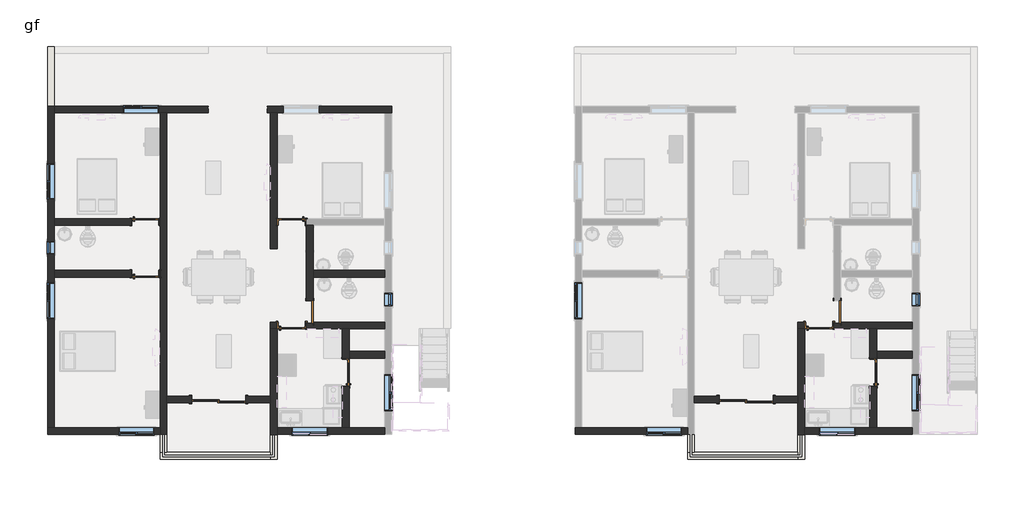
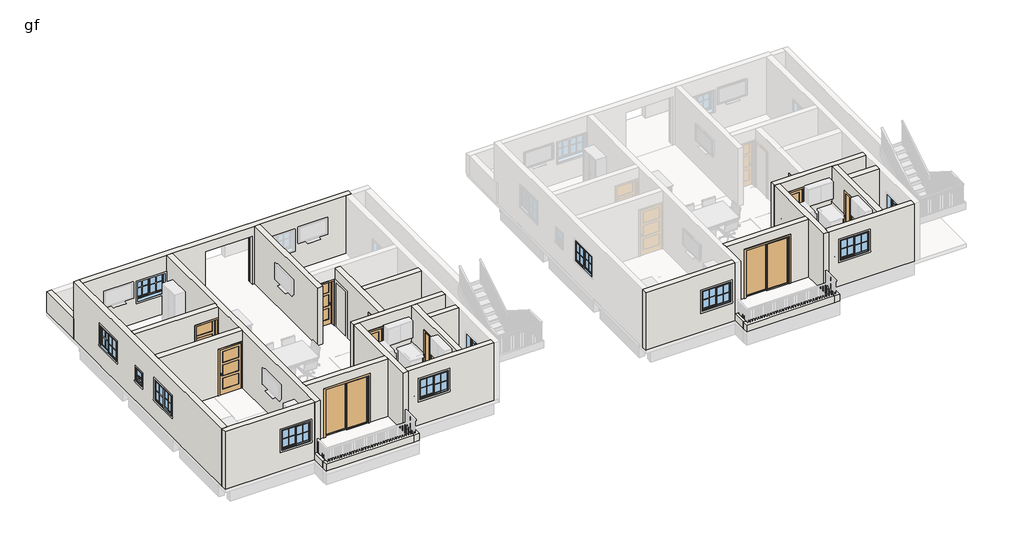
# One storey, part 1 of 8: 30 walls, 13 windows, 11 doors.
"""IFC4 building model written with IfcOpenShell, lengths in millimetres."""

from ifc_helpers import new_model, si_unit, frame, origin, place, context, project, spatial, polyline, outline, extrude, faceted_brep, transform, mapped, element, save
from components import door_d4d75d1e, door_2334f446, door_80766924, door_a1484949, window_608ea798, window_2eef0573, window_a5b1ea32

model = new_model("IFC4")

# Units and contexts
model_context = context("Model", 3, world=origin())
ifc_project = project(units=[si_unit("LENGTHUNIT", "METRE", prefix="MILLI")], contexts=[model_context])

# Site, building, storey
site = spatial("IfcSite", under=ifc_project)
building = spatial("IfcBuilding", under=site)
storey = spatial("IfcBuildingStorey", under=building, Name="gf", Elevation=609.6)

# Doors
placement = place(None, origin())
door_shape = door_d4d75d1e(model_context)
element("IfcDoor", 1, ObjectType="Door-Double-Sliding : 72\" x 84\"", at=placement, inside=storey, context=model_context, shape_type="MappedRepresentation", body=[
    mapped(door_shape, transform((-10509.3993763, -3297.2064015, 609.6), x_axis=(-1.0, 0.0, 0.0), y_axis=(0.0, -1.0, 0.0), z_axis=(0.0, 0.0, 1.0))),
])
element("IfcDoor", 2, ObjectType="Door-Double-Sliding : 72\" x 84\"", at=placement, inside=storey, context=model_context, shape_type="MappedRepresentation", body=[
    mapped(door_shape, transform((7365.1761273, -3297.2064015, 609.6), x_axis=(-1.0, 0.0, 0.0), y_axis=(0.0, -1.0, 0.0), z_axis=(0.0, 0.0, 1.0))),
])
door_2_shape = door_2334f446(model_context)
element("IfcDoor", 3, ObjectType="Door-Interior-Single-3_Panel_Vert-Wood : 36\" x 80\"", at=placement, inside=storey, context=model_context, shape_type="MappedRepresentation", body=[
    mapped(door_2_shape, transform((-12985.8993763, 2598.7685985, 609.6), x_axis=(1.0, 0.0, 0.0), y_axis=(0.0, 1.0, 0.0), z_axis=(0.0, 0.0, 1.0))),
])
door_3_shape = door_80766924(model_context)
element("IfcDoor", 4, ObjectType="Door-Interior-Single-3_Panel_Vert-Wood : 36\" x 80\"", at=placement, inside=storey, context=model_context, shape_type="MappedRepresentation", body=[
    mapped(door_3_shape, transform((-12985.8993763, 839.8185985, 609.6), x_axis=(1.0, 0.0, 0.0), y_axis=(0.0, 1.0, 0.0), z_axis=(0.0, 0.0, 1.0))),
])
element("IfcDoor", 5, ObjectType="Door-Interior-Single-3_Panel_Vert-Wood : 36\" x 80\"", at=placement, inside=storey, context=model_context, shape_type="MappedRepresentation", body=[
    mapped(door_3_shape, transform((-6200.9243763, -2509.8064015, 609.6), x_axis=(0.0, 1.0, 0.0), y_axis=(-1.0, 0.0, 0.0), z_axis=(0.0, 0.0, 1.0))),
])
element("IfcDoor", 6, ObjectType="Door-Interior-Single-3_Panel_Vert-Wood : 36\" x 80\"", at=placement, inside=storey, context=model_context, shape_type="MappedRepresentation", body=[
    mapped(door_3_shape, transform((-8032.8993763, -912.7814015, 609.6), x_axis=(1.0, 0.0, 0.0), y_axis=(0.0, 1.0, 0.0), z_axis=(0.0, 0.0, 1.0))),
])
element("IfcDoor", 7, ObjectType="Door-Interior-Single-3_Panel_Vert-Wood : 36\" x 80\"", at=placement, inside=storey, context=model_context, shape_type="MappedRepresentation", body=[
    mapped(door_3_shape, transform((-8032.8993763, 2598.7685985, 609.6), x_axis=(-1.0, 0.0, 0.0), y_axis=(0.0, -1.0, 0.0), z_axis=(0.0, 0.0, 1.0))),
])
element("IfcDoor", 8, ObjectType="Door-Interior-Single-3_Panel_Vert-Wood : 36\" x 80\"", at=placement, inside=storey, context=model_context, shape_type="MappedRepresentation", body=[
    mapped(door_3_shape, transform((11673.6511273, -2509.8064015, 609.6), x_axis=(0.0, 1.0, 0.0), y_axis=(-1.0, 0.0, 0.0), z_axis=(0.0, 0.0, 1.0))),
])
element("IfcDoor", 9, ObjectType="Door-Interior-Single-3_Panel_Vert-Wood : 36\" x 80\"", at=placement, inside=storey, context=model_context, shape_type="MappedRepresentation", body=[
    mapped(door_3_shape, transform((9841.6761273, -912.7814015, 609.6), x_axis=(1.0, 0.0, 0.0), y_axis=(0.0, 1.0, 0.0), z_axis=(0.0, 0.0, 1.0))),
])
door_4_shape = door_a1484949(model_context)
element("IfcDoor", 10, ObjectType="Single-Flush : 30\" x 80\"", at=placement, inside=storey, context=model_context, shape_type="MappedRepresentation", body=[
    mapped(door_4_shape, transform((-7423.2993763, -452.4064015, 609.6), x_axis=(0.0, -1.0, 0.0), y_axis=(1.0, 0.0, 0.0), z_axis=(0.0, 0.0, 1.0))),
])
element("IfcDoor", 11, ObjectType="Single-Flush : 30\" x 80\"", at=placement, inside=storey, context=model_context, shape_type="MappedRepresentation", body=[
    mapped(door_4_shape, transform((10451.2761273, -452.4064015, 609.6), x_axis=(0.0, -1.0, 0.0), y_axis=(1.0, 0.0, 0.0), z_axis=(0.0, 0.0, 1.0))),
])

# Walls
element("IfcWall", 12, at=placement, inside=storey, context=model_context, shape_type="Brep", body=[
    faceted_brep([(-16300.5993763, 6519.8935985, 609.6), (-16300.5993763, -4376.7064015, 609.6), (-16300.5993763, -4376.7064015, 3200.4), (-16300.5993763, 6519.8935985, 3200.4), (-16300.5993763, 4576.7935985, 2438.4), (-16300.5993763, 3357.5935985, 2438.4), (-16300.5993763, 3357.5935985, 1524.0), (-16300.5993763, 4576.7935985, 1524.0), (-16300.5993763, -681.0064015, 2438.4), (-16300.5993763, -681.0064015, 1524.0), (-16300.5993763, 538.1935985, 1524.0), (-16300.5993763, 538.1935985, 2438.4), (-16300.5993763, 1935.1935985, 2133.6), (-16300.5993763, 1503.3935985, 2133.6), (-16300.5993763, 1503.3935985, 1524.0), (-16300.5993763, 1935.1935985, 1524.0), (-16071.9993763, 6519.8935985, 609.6), (-16071.9993763, 6519.8935985, 3200.4), (-16071.9993763, 6291.2935985, 3200.4), (-16071.9993763, 2709.8935985, 3200.4), (-16071.9993763, 2481.2935985, 3200.4), (-16071.9993763, 957.2935985, 3200.4), (-16071.9993763, 728.6935985, 3200.4), (-16071.9993763, -4376.7064015, 3200.4), (-16071.9993763, -4376.7064015, 609.6), (-16071.9993763, 728.6935985, 609.6), (-16071.9993763, 957.2935985, 609.6), (-16071.9993763, 2481.2935985, 609.6), (-16071.9993763, 2709.8935985, 609.6), (-16071.9993763, 6291.2935985, 609.6), (-16071.9993763, 4576.7935985, 2438.4), (-16071.9993763, 4576.7935985, 1524.0), (-16071.9993763, 3357.5935985, 1524.0), (-16071.9993763, 3357.5935985, 2438.4), (-16071.9993763, -681.0064015, 2438.4), (-16071.9993763, 538.1935985, 2438.4), (-16071.9993763, 538.1935985, 1524.0), (-16071.9993763, -681.0064015, 1524.0), (-16071.9993763, 1935.1935985, 2133.6), (-16071.9993763, 1935.1935985, 1524.0), (-16071.9993763, 1503.3935985, 1524.0), (-16071.9993763, 1503.3935985, 2133.6)], [[[0, 1, 2, 3], [4, 5, 6, 7], [8, 9, 10, 11], [12, 13, 14, 15]], [[16, 17, 18, 19, 20, 21, 22, 23, 24, 25, 26, 27, 28, 29], [30, 31, 32, 33], [34, 35, 36, 37], [38, 39, 40, 41]], [[1, 0, 16, 29, 28, 27, 26, 25, 24]], [[3, 2, 23, 22, 21, 20, 19, 18, 17]], [[0, 3, 17, 16]], [[2, 1, 24, 23]], [[31, 30, 4, 7]], [[32, 31, 7, 6]], [[33, 32, 6, 5]], [[30, 33, 5, 4]], [[9, 8, 34, 37]], [[10, 9, 37, 36]], [[11, 10, 36, 35]], [[8, 11, 35, 34]], [[39, 38, 12, 15]], [[40, 39, 15, 14]], [[41, 40, 14, 13]], [[38, 41, 13, 12]]]),
])
element("IfcWall", 13, at=placement, inside=storey, context=model_context, shape_type="SweptSolid", body=[
    extrude(outline(polyline([(3200.4, -12490.5993763), (3200.4, -16071.9993763), (609.6, -16071.9993763), (609.6, -13468.4993763), (2667.0, -13468.4993763), (2667.0, -12503.2993763), (609.6, -12503.2993763), (609.6, -12490.5993763), (3200.4, -12490.5993763)])), frame((0.0, 2481.2935985, 0.0), z_axis=(0.0, 1.0, 0.0), x_axis=(0.0, 0.0, 1.0)), (0.0, 0.0, 1.0), 228.6),
])
element("IfcWall", 14, at=placement, inside=storey, context=model_context, shape_type="Brep", body=[
    faceted_brep([(-4641.9993763, 6291.2935985, 3200.4), (-4870.5993763, 6291.2935985, 3200.4), (-8528.1993763, 6291.2935985, 3200.4), (-8756.7993763, 6291.2935985, 3200.4), (-12261.9993763, 6291.2935985, 3200.4), (-12490.5993763, 6291.2935985, 3200.4), (-16071.9993763, 6291.2935985, 3200.4), (-16071.9993763, 6291.2935985, 609.6), (-12490.5993763, 6291.2935985, 609.6), (-12261.9993763, 6291.2935985, 609.6), (-10861.6993763, 6291.2935985, 609.6), (-10861.6993763, 6291.2935985, 2779.1), (-8861.6993763, 6291.2935985, 2779.1), (-8861.6993763, 6291.2935985, 609.6), (-8756.7993763, 6291.2935985, 609.6), (-8528.1993763, 6291.2935985, 609.6), (-4870.5993763, 6291.2935985, 609.6), (-4641.9993763, 6291.2935985, 609.6), (-8312.2993763, 6291.2935985, 2438.4), (-7093.0993763, 6291.2935985, 2438.4), (-7093.0993763, 6291.2935985, 1524.0), (-8312.2993763, 6291.2935985, 1524.0), (-12528.6993763, 6291.2935985, 2438.4), (-12528.6993763, 6291.2935985, 1524.0), (-13747.8993763, 6291.2935985, 1524.0), (-13747.8993763, 6291.2935985, 2438.4), (-16071.9993763, 6519.8935985, 3200.4), (-4641.9993763, 6519.8935985, 3200.4), (-4641.9993763, 6519.8935985, 609.6), (-8861.6993763, 6519.8935985, 609.6), (-8861.6993763, 6519.8935985, 2779.1), (-10861.6993763, 6519.8935985, 2779.1), (-10861.6993763, 6519.8935985, 609.6), (-16071.9993763, 6519.8935985, 609.6), (-8312.2993763, 6519.8935985, 2438.4), (-8312.2993763, 6519.8935985, 1524.0), (-7093.0993763, 6519.8935985, 1524.0), (-7093.0993763, 6519.8935985, 2438.4), (-12528.6993763, 6519.8935985, 2438.4), (-13747.8993763, 6519.8935985, 2438.4), (-13747.8993763, 6519.8935985, 1524.0), (-12528.6993763, 6519.8935985, 1524.0), (-10861.6993763, 6499.8935985, 609.6), (-10876.6993763, 6499.8935985, 609.6), (-10876.6993763, 6429.8935985, 609.6), (-10861.6993763, 6429.8935985, 609.6), (-8861.6993763, 6429.8935985, 609.6), (-8846.6993763, 6429.8935985, 609.6), (-8846.6993763, 6499.8935985, 609.6), (-8861.6993763, 6499.8935985, 609.6), (-8861.6993763, 6499.8935985, 2779.1), (-10861.6993763, 6499.8935985, 2779.1), (-10861.6993763, 6429.8935985, 2779.1), (-8861.6993763, 6429.8935985, 2779.1), (-10876.6993763, 6429.8935985, 2794.1), (-8846.6993763, 6429.8935985, 2794.1), (-8846.6993763, 6499.8935985, 2794.1), (-10876.6993763, 6499.8935985, 2794.1)], [[[0, 1, 2, 3, 4, 5, 6, 7, 8, 9, 10, 11, 12, 13, 14, 15, 16, 17], [18, 19, 20, 21], [22, 23, 24, 25]], [[26, 27, 28, 29, 30, 31, 32, 33], [34, 35, 36, 37], [38, 39, 40, 41]], [[7, 33, 32, 42, 43, 44, 45, 10, 9, 8]], [[28, 17, 16, 15, 14, 13, 46, 47, 48, 49, 29]], [[6, 5, 4, 3, 2, 1, 0, 27, 26]], [[7, 6, 26, 33]], [[0, 17, 28, 27]], [[50, 51, 31, 30]], [[52, 53, 12, 11]], [[45, 52, 11, 10]], [[53, 46, 13, 12]], [[53, 52, 45, 44, 54, 55, 47, 46]], [[47, 55, 56, 48]], [[51, 50, 49, 48, 56, 57, 43, 42]], [[49, 50, 30, 29]], [[51, 42, 32, 31]], [[54, 44, 43, 57]], [[55, 54, 57, 56]], [[35, 34, 18, 21]], [[36, 35, 21, 20]], [[37, 36, 20, 19]], [[34, 37, 19, 18]], [[23, 22, 38, 41]], [[24, 23, 41, 40]], [[25, 24, 40, 39]], [[22, 25, 39, 38]]]),
])
element("IfcWall", 15, at=placement, inside=storey, context=model_context, shape_type="Brep", body=[
    faceted_brep([(-4870.5993763, -4376.7064015, 609.6), (-6089.7993763, -4376.7064015, 609.6), (-6318.3993763, -4376.7064015, 609.6), (-8528.1993763, -4376.7064015, 609.6), (-8528.1993763, -4376.7064015, 3200.4), (-6318.3993763, -4376.7064015, 3200.4), (-6089.7993763, -4376.7064015, 3200.4), (-4870.5993763, -4376.7064015, 3200.4), (-8032.8993763, -4376.7064015, 2667.0), (-8032.8993763, -4376.7064015, 1752.6), (-6813.6993763, -4376.7064015, 1752.6), (-6813.6993763, -4376.7064015, 2667.0), (-4870.5993763, -4605.3064015, 609.6), (-4870.5993763, -4605.3064015, 3200.4), (-8528.1993763, -4605.3064015, 3200.4), (-8528.1993763, -4605.3064015, 609.6), (-8032.8993763, -4605.3064015, 2667.0), (-6813.6993763, -4605.3064015, 2667.0), (-6813.6993763, -4605.3064015, 1752.6), (-8032.8993763, -4605.3064015, 1752.6)], [[[0, 1, 2, 3, 4, 5, 6, 7], [8, 9, 10, 11]], [[12, 13, 14, 15], [16, 17, 18, 19]], [[3, 2, 1, 0, 12, 15]], [[7, 6, 5, 4, 14, 13]], [[0, 7, 13, 12]], [[4, 3, 15, 14]], [[9, 8, 16, 19]], [[10, 9, 19, 18]], [[11, 10, 18, 17]], [[8, 11, 17, 16]]]),
])
element("IfcWall", 16, at=placement, inside=storey, context=model_context, shape_type="Brep", body=[
    faceted_brep([(-8756.7993763, 6291.2935985, 609.6), (-8756.7993763, 1681.1935985, 609.6), (-8756.7993763, 1681.1935985, 3200.4), (-8756.7993763, 6291.2935985, 3200.4), (-8528.1993763, 6291.2935985, 609.6), (-8528.1993763, 6291.2935985, 3200.4), (-8528.1993763, 2709.8935985, 3200.4), (-8528.1993763, 2481.2935985, 3200.4), (-8528.1993763, 1681.1935985, 3200.4), (-8528.1993763, 1681.1935985, 609.6), (-8528.1993763, 2481.2935985, 609.6), (-8528.1993763, 2709.8935985, 609.6)], [[[0, 1, 2, 3]], [[4, 5, 6, 7, 8, 9, 10, 11]], [[1, 0, 4, 11, 10, 9]], [[2, 1, 9, 8]], [[3, 2, 8, 7, 6, 5]], [[0, 3, 5, 4]]]),
])
element("IfcWall", 17, at=placement, inside=storey, context=model_context, shape_type="Brep", body=[
    faceted_brep([(-8756.7993763, -5214.9064015, 609.6), (-12261.9993763, -5214.9064015, 609.6), (-12490.5993763, -5214.9064015, 609.6), (-12490.5993763, -5214.9064015, 914.4), (-12261.9993763, -5214.9064015, 914.4), (-8756.7993763, -5214.9064015, 914.4), (-8756.7993763, -5443.5064015, 609.6), (-8756.7993763, -5443.5064015, 914.4), (-12490.5993763, -5443.5064015, 914.4), (-12490.5993763, -5443.5064015, 609.6)], [[[0, 1, 2, 3, 4, 5]], [[6, 7, 8, 9]], [[2, 1, 0, 6, 9]], [[5, 4, 3, 8, 7]], [[0, 5, 7, 6]], [[3, 2, 9, 8]]]),
])
element("IfcWall", 18, at=placement, inside=storey, context=model_context, shape_type="SweptSolid", body=[
    extrude(outline(polyline([(-12261.9993763, -4611.6564015), (-12261.9993763, -5214.9064015), (-12490.5993763, -5214.9064015), (-12490.5993763, -4611.6564015), (-12261.9993763, -4611.6564015)])), frame((0.0, 0.0, 609.6), z_axis=(0.0, 0.0, 1.0), x_axis=(1.0, 0.0, 0.0)), (0.0, 0.0, 1.0), 304.8),
])
element("IfcWall", 19, at=placement, inside=storey, context=model_context, shape_type="Brep", body=[
    faceted_brep([(-16300.5993763, -4605.3064015, 609.6), (-12490.5993763, -4605.3064015, 609.6), (-12490.5993763, -4605.3064015, 3200.4), (-16300.5993763, -4605.3064015, 3200.4), (-13900.2993763, -4605.3064015, 2438.4), (-12681.0993763, -4605.3064015, 2438.4), (-12681.0993763, -4605.3064015, 1524.0), (-13900.2993763, -4605.3064015, 1524.0), (-16300.5993763, -4376.7064015, 609.6), (-16300.5993763, -4376.7064015, 3200.4), (-16071.9993763, -4376.7064015, 3200.4), (-12490.5993763, -4376.7064015, 3200.4), (-12490.5993763, -4376.7064015, 609.6), (-16071.9993763, -4376.7064015, 609.6), (-13900.2993763, -4376.7064015, 2438.4), (-13900.2993763, -4376.7064015, 1524.0), (-12681.0993763, -4376.7064015, 1524.0), (-12681.0993763, -4376.7064015, 2438.4)], [[[0, 1, 2, 3], [4, 5, 6, 7]], [[8, 9, 10, 11, 12, 13], [14, 15, 16, 17]], [[1, 0, 8, 13, 12]], [[3, 2, 11, 10, 9]], [[0, 3, 9, 8]], [[15, 14, 4, 7]], [[16, 15, 7, 6]], [[17, 16, 6, 5]], [[14, 17, 5, 4]], [[2, 1, 12, 11]]]),
])
element("IfcWall", 20, at=placement, inside=storey, context=model_context, shape_type="SweptSolid", body=[
    extrude(outline(polyline([(609.6, -12261.9993763), (609.6, -11423.7993763), (2743.2, -11423.7993763), (2743.2, -9594.9993763), (609.6, -9594.9993763), (609.6, -8756.7993763), (3200.4, -8756.7993763), (3200.4, -12261.9993763), (609.6, -12261.9993763)])), frame((0.0, -3538.5064015, 0.0), z_axis=(0.0, 1.0, 0.0), x_axis=(0.0, 0.0, 1.0)), (0.0, 0.0, 1.0), 228.6),
])
element("IfcWall", 21, at=placement, inside=storey, context=model_context, shape_type="Brep", body=[
    faceted_brep([(-8756.7993763, -795.3064015, 3200.4), (-7537.5993763, -795.3064015, 3200.4), (-7308.9993763, -795.3064015, 3200.4), (-4870.5993763, -795.3064015, 3200.4), (-4870.5993763, -795.3064015, 609.6), (-7308.9993763, -795.3064015, 609.6), (-7308.9993763, -795.3064015, 2641.6), (-7537.5993763, -795.3064015, 2641.6), (-7537.5993763, -795.3064015, 609.6), (-7550.2993763, -795.3064015, 609.6), (-7550.2993763, -795.3064015, 2667.0), (-8515.4993763, -795.3064015, 2667.0), (-8515.4993763, -795.3064015, 609.6), (-8756.7993763, -795.3064015, 609.6), (-4870.5993763, -1023.9064015, 3200.4), (-6089.7993763, -1023.9064015, 3200.4), (-6318.3993763, -1023.9064015, 3200.4), (-8528.1993763, -1023.9064015, 3200.4), (-8756.7993763, -1023.9064015, 3200.4), (-8756.7993763, -1023.9064015, 609.6), (-8528.1993763, -1023.9064015, 609.6), (-8515.4993763, -1023.9064015, 609.6), (-8515.4993763, -1023.9064015, 2667.0), (-7550.2993763, -1023.9064015, 2667.0), (-7550.2993763, -1023.9064015, 609.6), (-6318.3993763, -1023.9064015, 609.6), (-6089.7993763, -1023.9064015, 609.6), (-4870.5993763, -1023.9064015, 609.6), (-7537.5993763, -833.4064015, 609.6), (-7308.9993763, -833.4064015, 609.6), (-7537.5993763, -833.4064015, 2641.6), (-7308.9993763, -833.4064015, 2641.6)], [[[0, 1, 2, 3, 4, 5, 6, 7, 8, 9, 10, 11, 12, 13]], [[14, 15, 16, 17, 18, 19, 20, 21, 22, 23, 24, 25, 26, 27]], [[4, 27, 26, 25, 24, 9, 8, 28, 29, 5]], [[13, 12, 21, 20, 19]], [[3, 2, 1, 0, 18, 17, 16, 15, 14]], [[4, 3, 14, 27]], [[23, 10, 9, 24]], [[10, 23, 22, 11]], [[11, 22, 21, 12]], [[30, 28, 8, 7]], [[29, 31, 6, 5]], [[28, 30, 31, 29]], [[31, 30, 7, 6]], [[0, 13, 19, 18]]]),
])
element("IfcWall", 22, at=placement, inside=storey, context=model_context, shape_type="Brep", body=[
    faceted_brep([(-6318.3993763, -4376.7064015, 3200.4), (-6318.3993763, -1023.9064015, 3200.4), (-6318.3993763, -1023.9064015, 609.6), (-6318.3993763, -2027.2064015, 609.6), (-6318.3993763, -2027.2064015, 2667.0), (-6318.3993763, -2992.4064015, 2667.0), (-6318.3993763, -2992.4064015, 609.6), (-6318.3993763, -4376.7064015, 609.6), (-6089.7993763, -1023.9064015, 3200.4), (-6089.7993763, -1785.9064015, 3200.4), (-6089.7993763, -2014.5064015, 3200.4), (-6089.7993763, -4376.7064015, 3200.4), (-6089.7993763, -4376.7064015, 609.6), (-6089.7993763, -2992.4064015, 609.6), (-6089.7993763, -2992.4064015, 2667.0), (-6089.7993763, -2027.2064015, 2667.0), (-6089.7993763, -2027.2064015, 609.6), (-6089.7993763, -2014.5064015, 609.6), (-6089.7993763, -1785.9064015, 609.6), (-6089.7993763, -1023.9064015, 609.6)], [[[0, 1, 2, 3, 4, 5, 6, 7]], [[8, 9, 10, 11, 12, 13, 14, 15, 16, 17, 18, 19]], [[2, 19, 18, 17, 16, 3]], [[12, 7, 6, 13]], [[1, 0, 11, 10, 9, 8]], [[2, 1, 8, 19]], [[0, 7, 12, 11]], [[15, 4, 3, 16]], [[4, 15, 14, 5]], [[5, 14, 13, 6]]]),
])
element("IfcWall", 23, at=placement, inside=storey, context=model_context, shape_type="SweptSolid", body=[
    extrude(outline(polyline([(-4870.5993763, -2014.5064015), (-6089.7993763, -2014.5064015), (-6089.7993763, -1785.9064015), (-4870.5993763, -1785.9064015), (-4870.5993763, -2014.5064015)])), frame((0.0, 0.0, 609.6), z_axis=(0.0, 0.0, 1.0), x_axis=(1.0, 0.0, 0.0)), (0.0, 0.0, 1.0), 2590.8),
])
element("IfcWall", 24, at=placement, inside=storey, context=model_context, shape_type="SweptSolid", body=[
    extrude(outline(polyline([(-7308.9993763, 957.2935985), (-4870.5993763, 957.2935985), (-4870.5993763, 728.6935985), (-7308.9993763, 728.6935985), (-7308.9993763, 957.2935985)])), frame((0.0, 0.0, 609.6), z_axis=(0.0, 0.0, 1.0), x_axis=(1.0, 0.0, 0.0)), (0.0, 0.0, 1.0), 2590.8),
])
element("IfcWall", 25, at=placement, inside=storey, context=model_context, shape_type="Brep", body=[
    faceted_brep([(-7308.9993763, 2481.2935985, 3200.4), (-7308.9993763, 957.2935985, 3200.4), (-7308.9993763, 728.6935985, 3200.4), (-7308.9993763, -795.3064015, 3200.4), (-7308.9993763, -795.3064015, 2641.6), (-7308.9993763, -71.4064015, 2641.6), (-7308.9993763, -71.4064015, 609.6), (-7308.9993763, 728.6935985, 609.6), (-7308.9993763, 957.2935985, 609.6), (-7308.9993763, 2481.2935985, 609.6), (-7537.5993763, -795.3064015, 3200.4), (-7537.5993763, 2481.2935985, 3200.4), (-7537.5993763, 2481.2935985, 609.6), (-7537.5993763, -71.4064015, 609.6), (-7537.5993763, -71.4064015, 2641.6), (-7537.5993763, -795.3064015, 2641.6)], [[[0, 1, 2, 3, 4, 5, 6, 7, 8, 9]], [[10, 11, 12, 13, 14, 15]], [[12, 9, 8, 7, 6, 13]], [[3, 2, 1, 0, 11, 10]], [[3, 10, 15, 4]], [[0, 9, 12, 11]], [[14, 5, 4, 15]], [[5, 14, 13, 6]]]),
])
element("IfcWall", 26, at=placement, inside=storey, context=model_context, shape_type="SweptSolid", body=[
    extrude(outline(polyline([(2481.2935985, 609.6), (2405.0935985, 609.6), (2405.0935985, 2641.6), (1643.0935985, 2641.6), (1643.0935985, 609.6), (957.2935985, 609.6), (957.2935985, 3200.4), (2481.2935985, 3200.4), (2481.2935985, 609.6)])), frame((-7537.5993763, 0.0, 0.0), z_axis=(1.0, 0.0, 0.0), x_axis=(0.0, 1.0, 0.0)), (0.0, 0.0, 1.0), 228.6),
])
element("IfcWall", 27, at=placement, inside=storey, context=model_context, shape_type="SweptSolid", body=[
    extrude(outline(polyline([(3200.4, -12490.5993763), (3200.4, -16071.9993763), (609.6, -16071.9993763), (609.6, -13468.4993763), (2667.0, -13468.4993763), (2667.0, -12503.2993763), (609.6, -12503.2993763), (609.6, -12490.5993763), (3200.4, -12490.5993763)])), frame((0.0, 728.6935985, 0.0), z_axis=(0.0, 1.0, 0.0), x_axis=(0.0, 0.0, 1.0)), (0.0, 0.0, 1.0), 228.6),
])
element("IfcWall", 28, at=placement, inside=storey, context=model_context, shape_type="Brep", body=[
    faceted_brep([(-8756.7993763, -1023.9064015, 609.6), (-8756.7993763, -3309.9064015, 609.6), (-8756.7993763, -3538.5064015, 609.6), (-8756.7993763, -4618.0064015, 609.6), (-8756.7993763, -4618.0064015, 914.4), (-8756.7993763, -4618.0064015, 3200.4), (-8756.7993763, -3538.5064015, 3200.4), (-8756.7993763, -3309.9064015, 3200.4), (-8756.7993763, -1023.9064015, 3200.4), (-8528.1993763, -1023.9064015, 609.6), (-8528.1993763, -1023.9064015, 3200.4), (-8528.1993763, -4376.7064015, 3200.4), (-8528.1993763, -4605.3064015, 3200.4), (-8528.1993763, -4618.0064015, 3200.4), (-8528.1993763, -4618.0064015, 914.4), (-8528.1993763, -4618.0064015, 609.6), (-8528.1993763, -4605.3064015, 609.6), (-8528.1993763, -4376.7064015, 609.6)], [[[0, 1, 2, 3, 4, 5, 6, 7, 8]], [[9, 10, 11, 12, 13, 14, 15, 16, 17]], [[3, 2, 1, 0, 9, 17, 16, 15]], [[5, 4, 3, 15, 14, 13]], [[8, 7, 6, 5, 13, 12, 11, 10]], [[0, 8, 10, 9]]]),
])
element("IfcWall", 29, at=placement, inside=storey, context=model_context, shape_type="Brep", body=[
    faceted_brep([(-12261.9993763, -4605.3064015, 609.6), (-12261.9993763, -3538.5064015, 609.6), (-12261.9993763, -3309.9064015, 609.6), (-12261.9993763, 6291.2935985, 609.6), (-12261.9993763, 6291.2935985, 3200.4), (-12261.9993763, -3309.9064015, 3200.4), (-12261.9993763, -3538.5064015, 3200.4), (-12261.9993763, -4605.3064015, 3200.4), (-12490.5993763, -4605.3064015, 609.6), (-12490.5993763, -4605.3064015, 3200.4), (-12490.5993763, -4376.7064015, 3200.4), (-12490.5993763, 728.6935985, 3200.4), (-12490.5993763, 957.2935985, 3200.4), (-12490.5993763, 2481.2935985, 3200.4), (-12490.5993763, 2709.8935985, 3200.4), (-12490.5993763, 6291.2935985, 3200.4), (-12490.5993763, 6291.2935985, 609.6), (-12490.5993763, 2709.8935985, 609.6), (-12490.5993763, 2481.2935985, 609.6), (-12490.5993763, 957.2935985, 609.6), (-12490.5993763, 728.6935985, 609.6), (-12490.5993763, -4376.7064015, 609.6)], [[[0, 1, 2, 3, 4, 5, 6, 7]], [[8, 9, 10, 11, 12, 13, 14, 15, 16, 17, 18, 19, 20, 21]], [[3, 2, 1, 0, 8, 21, 20, 19, 18, 17, 16]], [[7, 6, 5, 4, 15, 14, 13, 12, 11, 10, 9]], [[4, 3, 16, 15]], [[0, 7, 9, 8]]]),
])
element("IfcWall", 30, at=placement, inside=storey, context=model_context, shape_type="Brep", body=[
    faceted_brep([(-8756.7993763, -4618.0064015, 609.6), (-8756.7993763, -5214.9064015, 609.6), (-8756.7993763, -5443.5064015, 609.6), (-8756.7993763, -5443.5064015, 914.4), (-8756.7993763, -5214.9064015, 914.4), (-8756.7993763, -4618.0064015, 914.4), (-8528.1993763, -4618.0064015, 609.6), (-8528.1993763, -4618.0064015, 914.4), (-8528.1993763, -5443.5064015, 914.4), (-8528.1993763, -5443.5064015, 609.6)], [[[0, 1, 2, 3, 4, 5]], [[6, 7, 8, 9]], [[2, 1, 0, 6, 9]], [[5, 4, 3, 8, 7]], [[0, 5, 7, 6]], [[3, 2, 9, 8]]]),
])
element("IfcWall", 31, at=placement, inside=storey, context=model_context, shape_type="Brep", body=[
    faceted_brep([(13003.9761273, -4376.7064015, 609.6), (11784.7761273, -4376.7064015, 609.6), (11556.1761273, -4376.7064015, 609.6), (9346.3761273, -4376.7064015, 609.6), (9346.3761273, -4376.7064015, 3200.4), (11556.1761273, -4376.7064015, 3200.4), (11784.7761273, -4376.7064015, 3200.4), (13003.9761273, -4376.7064015, 3200.4), (9841.6761273, -4376.7064015, 2667.0), (9841.6761273, -4376.7064015, 1752.6), (11060.8761273, -4376.7064015, 1752.6), (11060.8761273, -4376.7064015, 2667.0), (13003.9761273, -4605.3064015, 609.6), (13003.9761273, -4605.3064015, 3200.4), (9346.3761273, -4605.3064015, 3200.4), (9346.3761273, -4605.3064015, 609.6), (9841.6761273, -4605.3064015, 2667.0), (11060.8761273, -4605.3064015, 2667.0), (11060.8761273, -4605.3064015, 1752.6), (9841.6761273, -4605.3064015, 1752.6)], [[[0, 1, 2, 3, 4, 5, 6, 7], [8, 9, 10, 11]], [[12, 13, 14, 15], [16, 17, 18, 19]], [[3, 2, 1, 0, 12, 15]], [[7, 6, 5, 4, 14, 13]], [[4, 3, 15, 14]], [[9, 8, 16, 19]], [[10, 9, 19, 18]], [[11, 10, 18, 17]], [[8, 11, 17, 16]], [[0, 7, 13, 12]]]),
])
element("IfcWall", 32, at=placement, inside=storey, context=model_context, shape_type="Brep", body=[
    faceted_brep([(9117.7761273, -5214.9064015, 609.6), (5612.5761273, -5214.9064015, 609.6), (5383.9761273, -5214.9064015, 609.6), (5383.9761273, -5214.9064015, 914.4), (5612.5761273, -5214.9064015, 914.4), (9117.7761273, -5214.9064015, 914.4), (9117.7761273, -5443.5064015, 609.6), (9117.7761273, -5443.5064015, 914.4), (5383.9761273, -5443.5064015, 914.4), (5383.9761273, -5443.5064015, 609.6)], [[[0, 1, 2, 3, 4, 5]], [[6, 7, 8, 9]], [[2, 1, 0, 6, 9]], [[5, 4, 3, 8, 7]], [[0, 5, 7, 6]], [[3, 2, 9, 8]]]),
])
element("IfcWall", 33, at=placement, inside=storey, context=model_context, shape_type="SweptSolid", body=[
    extrude(outline(polyline([(5612.5761273, -4611.6564015), (5612.5761273, -5214.9064015), (5383.9761273, -5214.9064015), (5383.9761273, -4611.6564015), (5612.5761273, -4611.6564015)])), frame((0.0, 0.0, 609.6), z_axis=(0.0, 0.0, 1.0), x_axis=(1.0, 0.0, 0.0)), (0.0, 0.0, 1.0), 304.8),
])
element("IfcWall", 34, at=placement, inside=storey, context=model_context, shape_type="Brep", body=[
    faceted_brep([(1573.9761273, -4605.3064015, 609.6), (5383.9761273, -4605.3064015, 609.6), (5383.9761273, -4605.3064015, 3200.4), (1573.9761273, -4605.3064015, 3200.4), (3974.2761273, -4605.3064015, 2438.4), (5193.4761273, -4605.3064015, 2438.4), (5193.4761273, -4605.3064015, 1524.0), (3974.2761273, -4605.3064015, 1524.0), (1573.9761273, -4376.7064015, 609.6), (1573.9761273, -4376.7064015, 3200.4), (1802.5761273, -4376.7064015, 3200.4), (5383.9761273, -4376.7064015, 3200.4), (5383.9761273, -4376.7064015, 609.6), (1802.5761273, -4376.7064015, 609.6), (3974.2761273, -4376.7064015, 2438.4), (3974.2761273, -4376.7064015, 1524.0), (5193.4761273, -4376.7064015, 1524.0), (5193.4761273, -4376.7064015, 2438.4)], [[[0, 1, 2, 3], [4, 5, 6, 7]], [[8, 9, 10, 11, 12, 13], [14, 15, 16, 17]], [[1, 0, 8, 13, 12]], [[3, 2, 11, 10, 9]], [[0, 3, 9, 8]], [[15, 14, 4, 7]], [[16, 15, 7, 6]], [[17, 16, 6, 5]], [[14, 17, 5, 4]], [[2, 1, 12, 11]]]),
])
element("IfcWall", 35, at=placement, inside=storey, context=model_context, shape_type="SweptSolid", body=[
    extrude(outline(polyline([(609.6, 5612.5761273), (609.6, 6450.7761273), (2743.2, 6450.7761273), (2743.2, 8279.5761273), (609.6, 8279.5761273), (609.6, 9117.7761273), (3200.4, 9117.7761273), (3200.4, 5612.5761273), (609.6, 5612.5761273)])), frame((0.0, -3538.5064015, 0.0), z_axis=(0.0, 1.0, 0.0), x_axis=(0.0, 0.0, 1.0)), (0.0, 0.0, 1.0), 228.6),
])
element("IfcWall", 36, at=placement, inside=storey, context=model_context, shape_type="Brep", body=[
    faceted_brep([(9117.7761273, -795.3064015, 3200.4), (10336.9761273, -795.3064015, 3200.4), (10565.5761273, -795.3064015, 3200.4), (13003.9761273, -795.3064015, 3200.4), (13003.9761273, -795.3064015, 609.6), (10565.5761273, -795.3064015, 609.6), (10565.5761273, -795.3064015, 2641.6), (10336.9761273, -795.3064015, 2641.6), (10336.9761273, -795.3064015, 609.6), (10324.2761273, -795.3064015, 609.6), (10324.2761273, -795.3064015, 2667.0), (9359.0761273, -795.3064015, 2667.0), (9359.0761273, -795.3064015, 609.6), (9117.7761273, -795.3064015, 609.6), (13003.9761273, -1023.9064015, 3200.4), (11784.7761273, -1023.9064015, 3200.4), (11556.1761273, -1023.9064015, 3200.4), (9346.3761273, -1023.9064015, 3200.4), (9117.7761273, -1023.9064015, 3200.4), (9117.7761273, -1023.9064015, 609.6), (9346.3761273, -1023.9064015, 609.6), (9359.0761273, -1023.9064015, 609.6), (9359.0761273, -1023.9064015, 2667.0), (10324.2761273, -1023.9064015, 2667.0), (10324.2761273, -1023.9064015, 609.6), (11556.1761273, -1023.9064015, 609.6), (11784.7761273, -1023.9064015, 609.6), (13003.9761273, -1023.9064015, 609.6), (10336.9761273, -833.4064015, 609.6), (10565.5761273, -833.4064015, 609.6), (10336.9761273, -833.4064015, 2641.6), (10565.5761273, -833.4064015, 2641.6)], [[[0, 1, 2, 3, 4, 5, 6, 7, 8, 9, 10, 11, 12, 13]], [[14, 15, 16, 17, 18, 19, 20, 21, 22, 23, 24, 25, 26, 27]], [[4, 27, 26, 25, 24, 9, 8, 28, 29, 5]], [[13, 12, 21, 20, 19]], [[3, 2, 1, 0, 18, 17, 16, 15, 14]], [[4, 3, 14, 27]], [[23, 10, 9, 24]], [[10, 23, 22, 11]], [[11, 22, 21, 12]], [[30, 28, 8, 7]], [[29, 31, 6, 5]], [[28, 30, 31, 29]], [[31, 30, 7, 6]], [[0, 13, 19, 18]]]),
])
element("IfcWall", 37, at=placement, inside=storey, context=model_context, shape_type="Brep", body=[
    faceted_brep([(11556.1761273, -4376.7064015, 3200.4), (11556.1761273, -1023.9064015, 3200.4), (11556.1761273, -1023.9064015, 609.6), (11556.1761273, -2027.2064015, 609.6), (11556.1761273, -2027.2064015, 2667.0), (11556.1761273, -2992.4064015, 2667.0), (11556.1761273, -2992.4064015, 609.6), (11556.1761273, -4376.7064015, 609.6), (11784.7761273, -1023.9064015, 3200.4), (11784.7761273, -1785.9064015, 3200.4), (11784.7761273, -2014.5064015, 3200.4), (11784.7761273, -4376.7064015, 3200.4), (11784.7761273, -4376.7064015, 609.6), (11784.7761273, -2992.4064015, 609.6), (11784.7761273, -2992.4064015, 2667.0), (11784.7761273, -2027.2064015, 2667.0), (11784.7761273, -2027.2064015, 609.6), (11784.7761273, -2014.5064015, 609.6), (11784.7761273, -1785.9064015, 609.6), (11784.7761273, -1023.9064015, 609.6)], [[[0, 1, 2, 3, 4, 5, 6, 7]], [[8, 9, 10, 11, 12, 13, 14, 15, 16, 17, 18, 19]], [[2, 19, 18, 17, 16, 3]], [[12, 7, 6, 13]], [[1, 0, 11, 10, 9, 8]], [[2, 1, 8, 19]], [[0, 7, 12, 11]], [[15, 4, 3, 16]], [[4, 15, 14, 5]], [[5, 14, 13, 6]]]),
])
element("IfcWall", 38, at=placement, inside=storey, context=model_context, shape_type="SweptSolid", body=[
    extrude(outline(polyline([(13003.9761273, -2014.5064015), (11784.7761273, -2014.5064015), (11784.7761273, -1785.9064015), (13003.9761273, -1785.9064015), (13003.9761273, -2014.5064015)])), frame((0.0, 0.0, 609.6), z_axis=(0.0, 0.0, 1.0), x_axis=(1.0, 0.0, 0.0)), (0.0, 0.0, 1.0), 2590.8),
])
element("IfcWall", 39, at=placement, inside=storey, context=model_context, shape_type="Brep", body=[
    faceted_brep([(9117.7761273, -1023.9064015, 609.6), (9117.7761273, -3309.9064015, 609.6), (9117.7761273, -3538.5064015, 609.6), (9117.7761273, -4618.0064015, 609.6), (9117.7761273, -4618.0064015, 914.4), (9117.7761273, -4618.0064015, 3200.4), (9117.7761273, -3538.5064015, 3200.4), (9117.7761273, -3309.9064015, 3200.4), (9117.7761273, -1023.9064015, 3200.4), (9346.3761273, -1023.9064015, 609.6), (9346.3761273, -1023.9064015, 3200.4), (9346.3761273, -4376.7064015, 3200.4), (9346.3761273, -4605.3064015, 3200.4), (9346.3761273, -4618.0064015, 3200.4), (9346.3761273, -4618.0064015, 914.4), (9346.3761273, -4618.0064015, 609.6), (9346.3761273, -4605.3064015, 609.6), (9346.3761273, -4376.7064015, 609.6)], [[[0, 1, 2, 3, 4, 5, 6, 7, 8]], [[9, 10, 11, 12, 13, 14, 15, 16, 17]], [[3, 2, 1, 0, 9, 17, 16, 15]], [[5, 4, 3, 15, 14, 13]], [[8, 7, 6, 5, 13, 12, 11, 10]], [[0, 8, 10, 9]]]),
])
element("IfcWall", 40, at=placement, inside=storey, context=model_context, shape_type="Brep", body=[
    faceted_brep([(9117.7761273, -4618.0064015, 609.6), (9117.7761273, -5214.9064015, 609.6), (9117.7761273, -5443.5064015, 609.6), (9117.7761273, -5443.5064015, 914.4), (9117.7761273, -5214.9064015, 914.4), (9117.7761273, -4618.0064015, 914.4), (9346.3761273, -4618.0064015, 609.6), (9346.3761273, -4618.0064015, 914.4), (9346.3761273, -5443.5064015, 914.4), (9346.3761273, -5443.5064015, 609.6)], [[[0, 1, 2, 3, 4, 5]], [[6, 7, 8, 9]], [[2, 1, 0, 6, 9]], [[5, 4, 3, 8, 7]], [[0, 5, 7, 6]], [[3, 2, 9, 8]]]),
])
element("IfcWall", 41, at=placement, inside=storey, context=model_context, shape_type="Brep", body=[
    faceted_brep([(-16071.9993763, 6526.2435985, 609.6), (-16071.9993763, 8310.5935985, 609.6), (-16071.9993763, 8539.1935985, 609.6), (-16071.9993763, 8539.1935985, 1524.0), (-16071.9993763, 8310.5935985, 1524.0), (-16071.9993763, 6526.2435985, 1524.0), (-16300.5993763, 6526.2435985, 609.6), (-16300.5993763, 6526.2435985, 1524.0), (-16300.5993763, 8539.1935985, 1524.0), (-16300.5993763, 8539.1935985, 609.6)], [[[0, 1, 2, 3, 4, 5]], [[6, 7, 8, 9]], [[2, 1, 0, 6, 9]], [[5, 4, 3, 8, 7]], [[0, 5, 7, 6]], [[3, 2, 9, 8]]]),
])

# Windows
window_shape = window_608ea798(model_context)
element("IfcWindow", 42, ObjectType="Window-Fixed-Transom : 17\" x 24\"", at=placement, inside=storey, context=model_context, shape_type="MappedRepresentation", body=[
    mapped(window_shape, transform((-4756.2993763, -33.3064015, 609.6), x_axis=(0.0, -1.0, 0.0), y_axis=(1.0, 0.0, 0.0), z_axis=(0.0, 0.0, 1.0))),
])
element("IfcWindow", 43, ObjectType="Window-Fixed-Transom : 17\" x 24\"", at=placement, inside=storey, context=model_context, shape_type="MappedRepresentation", body=[
    mapped(window_shape, transform((-16186.2993763, 1719.2935985, 609.6), x_axis=(0.0, 1.0, 0.0), y_axis=(-1.0, 0.0, 0.0), z_axis=(0.0, 0.0, 1.0))),
])
element("IfcWindow", 44, ObjectType="Window-Fixed-Transom : 17\" x 24\"", at=placement, inside=storey, context=model_context, shape_type="MappedRepresentation", body=[
    mapped(window_shape, transform((13118.2761273, -33.3064015, 609.6), x_axis=(0.0, -1.0, 0.0), y_axis=(1.0, 0.0, 0.0), z_axis=(0.0, 0.0, 1.0))),
])
window_2_shape = window_2eef0573(model_context)
element("IfcWindow", 45, ObjectType="Window-Sliding-Double : 48\" x 36\"", at=placement, inside=storey, context=model_context, shape_type="MappedRepresentation", body=[
    mapped(window_2_shape, transform((-7423.2993763, -4494.8164015, 838.2), x_axis=(-1.0, 0.0, 0.0), y_axis=(0.0, -1.0, 0.0), z_axis=(0.0, 0.0, 1.0))),
])
element("IfcWindow", 46, ObjectType="Window-Sliding-Double : 48\" x 36\"", at=placement, inside=storey, context=model_context, shape_type="MappedRepresentation", body=[
    mapped(window_2_shape, transform((-13138.2993763, 6409.4035985, 609.6), x_axis=(1.0, 0.0, 0.0), y_axis=(0.0, 1.0, 0.0), z_axis=(0.0, 0.0, 1.0))),
])
element("IfcWindow", 47, ObjectType="Window-Sliding-Double : 48\" x 36\"", at=placement, inside=storey, context=model_context, shape_type="MappedRepresentation", body=[
    mapped(window_2_shape, transform((-16190.1093763, 3967.1935985, 609.6), x_axis=(0.0, 1.0, 0.0), y_axis=(-1.0, 0.0, 0.0), z_axis=(0.0, 0.0, 1.0))),
])
element("IfcWindow", 48, ObjectType="Window-Sliding-Double : 48\" x 36\"", at=placement, inside=storey, context=model_context, shape_type="MappedRepresentation", body=[
    mapped(window_2_shape, transform((-13290.6993763, -4494.8164015, 609.6), x_axis=(-1.0, 0.0, 0.0), y_axis=(0.0, -1.0, 0.0), z_axis=(0.0, 0.0, 1.0))),
])
element("IfcWindow", 49, ObjectType="Window-Sliding-Double : 48\" x 36\"", at=placement, inside=storey, context=model_context, shape_type="MappedRepresentation", body=[
    mapped(window_2_shape, transform((-4752.4893763, -3195.6064015, 609.6), x_axis=(0.0, -1.0, 0.0), y_axis=(1.0, 0.0, 0.0), z_axis=(0.0, 0.0, 1.0))),
])
element("IfcWindow", 50, ObjectType="Window-Sliding-Double : 48\" x 36\"", at=placement, inside=storey, context=model_context, shape_type="MappedRepresentation", body=[
    mapped(window_2_shape, transform((10451.2761273, -4494.8164015, 838.2), x_axis=(-1.0, 0.0, 0.0), y_axis=(0.0, -1.0, 0.0), z_axis=(0.0, 0.0, 1.0))),
])
element("IfcWindow", 51, ObjectType="Window-Sliding-Double : 48\" x 36\"", at=placement, inside=storey, context=model_context, shape_type="MappedRepresentation", body=[
    mapped(window_2_shape, transform((4583.8761273, -4494.8164015, 609.6), x_axis=(-1.0, 0.0, 0.0), y_axis=(0.0, -1.0, 0.0), z_axis=(0.0, 0.0, 1.0))),
])
element("IfcWindow", 52, ObjectType="Window-Sliding-Double : 48\" x 36\"", at=placement, inside=storey, context=model_context, shape_type="MappedRepresentation", body=[
    mapped(window_2_shape, transform((13122.0861273, -3195.6064015, 609.6), x_axis=(0.0, -1.0, 0.0), y_axis=(1.0, 0.0, 0.0), z_axis=(0.0, 0.0, 1.0))),
])
window_3_shape = window_a5b1ea32(model_context)
element("IfcWindow", 53, ObjectType="Window-Sliding-Double : 48\" x 36\"", at=placement, inside=storey, context=model_context, shape_type="MappedRepresentation", body=[
    mapped(window_3_shape, transform((-16190.1093763, -71.4064015, 609.6), x_axis=(0.0, -1.0, 0.0), y_axis=(1.0, 0.0, 0.0), z_axis=(0.0, 0.0, 1.0))),
])
element("IfcWindow", 54, ObjectType="Window-Sliding-Double : 48\" x 36\"", at=placement, inside=storey, context=model_context, shape_type="MappedRepresentation", body=[
    mapped(window_3_shape, transform((1684.4661273, -71.4064015, 609.6), x_axis=(0.0, -1.0, 0.0), y_axis=(1.0, 0.0, 0.0), z_axis=(0.0, 0.0, 1.0))),
])

save(model, "model.ifc")

# Revit data of these elements
# Type "Door-Double-Sliding : 72\" x 84\""
#   Type Mark = "13"
#   Construction Type Id = "opn-d45"
#   Assembly Code = "C1020"
#   Analytic Construction = "Wood frame, double glass door "
#   Thickness = 0' - 2"
#   Thermal Resistance (R) = 1.8150 (h·ft²·°F)/BTU
#   Heat Transfer Coefficient (U) = 0.5510 BTU/(h·ft²·°F)
#   Height = 7' - 0"
#   Rail Width = 0' - 2"
#   Stiles = 0' - 2"
#   Trim Projection Ext = 0' - 1"
#   Trim Projection Int = 0' - 1"
#   Trim Width = 0' - 3"
#   Width = 6' - 0"
#   Define Thermal Properties by = 1
#   Glazing = Glass
#   Panel Material = Wood - Birch - Solid Stained Light Low Gloss
#   Trim Material = Paint - Sienna
#   Visual Light Transmittance = 0
#   Solar Heat Gain Coefficient = 0
#   Function = (empty or 0)
#   Wall Closure = (empty or 0)
# Type "Door-Interior-Single-3_Panel_Vert-Wood : 36\" x 80\""
#   Type Mark = "10"
#   Assembly Code = "C1020300"
#   Analytic Construction = "Wooden"
#   Top Rail = 0' - 4 11/16"
#   Thickness = 0' - 1 3/8"
#   Thermal Resistance (R) = 2.5876 (h·ft²·°F)/BTU
#   Swing Angle [instance default] = 90.00°
#   Stiles = 0' - 4 3/4"
#   Rough Width = 3' - 2"
#   Rough Height = 6' - 9"
#   Intermediate Rail = 0' - 4 1/2"
#   Height = 6' - 8"
#   Width = 3' - 0"
#   Heat Transfer Coefficient (U) = 0.3865 BTU/(h·ft²·°F)
#   Bottom Rail = 0' - 9 1/8"
#   Trim Material = Cherry
#   Panel Material = Cherry
#   Frame Material = Cherry
#   Door Handle Material = Aluminum
#   Visual Light Transmittance = 0
#   Solar Heat Gain Coefficient = 0
#   Wall Closure = (empty or 0)
#   Function = (empty or 0)
# Type "Single-Flush : 30\" x 80\""
#   Type Mark = "5"
#   Construction Type Id = "MDOOR"
#   Assembly Code = "C1020"
#   Analytic Construction = "Metal"
#   Thickness = 0' - 2"
#   Heat Transfer Coefficient (U) = 0.651978 BTU/(h·ft²·°F)
#   Height = 6' - 8"
#   Trim Projection Ext = 0' - 1"
#   Trim Projection Int = 0' - 1"
#   Trim Width = 0' - 3"
#   Width = 2' - 6"
#   Define Thermal Properties by = 1
#   Define Thermal Properties by = 1
#   Door Material = Door - Panel
#   Frame Material = Door - Frame
#   Visual Light Transmittance = 0
#   Solar Heat Gain Coefficient = 0
#   Function = (empty or 0)
#   Wall Closure = (empty or 0)
# Type
#   Assembly Code = "B2010"
#   Layers, outside or top first: 0' - 9" no material (function 1)
# Type "Window-Fixed-Transom : 17\" x 24\""
#   Type Mark = "19"
#   Fire Rating = "0.5h"
#   Assembly Code = "B2020100"
#   Analytic Construction = "Double glazing - domestic"
#   Window Inset [instance default] = 0' - 0"
#   Wall Thickness [instance default] = 0' - 6"
#   Visual Light Transmittance = 0.81
#   Transom Height = 1' - 0"
#   Thermal Resistance (R) = 1.8146 (h·ft²·°F)/BTU
#   Solar Heat Gain Coefficient = 0.76
#   Rough Width = 1' - 5 1/2"
#   Rough Height = 2' - 0 1/2"
#   Lower Sash Height = 1' - 0"
#   Interior Wall Closure [instance default] = 0' - 2 1/4"
#   Height = 2' - 0"
#   Heat Transfer Coefficient (U) = 0.5511 BTU/(h·ft²·°F)
#   Frame Extension [instance default] = 0' - 0 1/4"
#   Exterior Wall Closure [instance default] = 0' - 1 1/4"
#   Extension Jamb [instance default] = 0' - 2 1/4"
#   Default Sill Height = 3' - 0"
#   Width = 1' - 5"
#   Muntin Visibility = yes
#   Interior Trim Visibility [instance default] = yes
#   Exterior Trim Visibility [instance default] = yes
#   Extension Jamb Visibility [instance default] = yes
#   Muntin Pattern = Muntin Pattern_2x2 : Muntin Pattern_2x2
#   Interior Trim Material = Wood - Stained
#   Interior Trim = Trim-Window-Interior-Flat : Picture Frame
#   Interior Frame Material = Wood - Stained
#   Glass Panel Material = Glass
#   Exterior Trim Material = Clad - White
#   Exterior Trim = Trim-Window-Exterior-Flat : with Sill
#   Exterior Frame Material = Clad - White
#   Wall Closure = (empty or 0)
# Type "Window-Sliding-Double : 48\" x 36\""
#   Type Mark = "18"
#   Fire Rating = "0.5h"
#   Assembly Code = "B2020100"
#   Analytic Construction = "Double glazing - domestic"
#   Window Inset [instance default] = 0' - 0"
#   Wall Thickness [instance default] = 0' - 6"
#   Visual Light Transmittance = 0.81
#   Thermal Resistance (R) = 1.8146 (h·ft²·°F)/BTU
#   Solar Heat Gain Coefficient = 0.76
#   Muntin Width = 1' - 8 5/8"
#   Muntin Height = 2' - 6 1/4"
#   Interior Wall Closure [instance default] = 0' - 2 3/4"
#   Heat Transfer Coefficient (U) = 0.5511 BTU/(h·ft²·°F)
#   Frame Extension [instance default] = 0' - 0 1/4"
#   Exterior Wall Closure [instance default] = 0' - 1 1/4"
#   Rough Width = 4' - 0 1/2"
#   Rough Height = 3' - 0 1/2"
#   Height = 3' - 0"
#   Extension Jamb [instance default] = 0' - 2 3/4"
#   Default Sill Height = 3' - 0"
#   Width = 4' - 0"
#   Interior Trim Visibility [instance default] = yes
#   Indicator Visibility [instance default] = yes
#   Exterior Trim Visibility [instance default] = yes
#   Muntin Visibility = yes
#   Extension Jamb Visibility [instance default] = yes
#   Muntin Pattern = Muntin Pattern_2x2 : Muntin Pattern_2x2
#   Interior Trim Material = Wood - Stained
#   Interior Trim = Trim-Window-Interior-Flat : Picture Frame
#   Interior Frame Material = Wood - Stained
#   Glass Panel Material = Glass
#   Exterior Trim Material = Clad - White
#   Exterior Trim = Trim-Window-Exterior-Flat : with Sill
#   Exterior Frame Material = Clad - White
#   Wall Closure = (empty or 0)
# Elements 1, 2 (IfcDoor, "Door-Double-Sliding : 72\" x 84\"")
#   Phase Created = New Construction
#   Materials on its faces: "Paint - Sienna", "Wood - Birch - Solid Stained Light Low Gloss", "Glass"
# Elements 3, 4, 5, 6, 7, 8, 9 (IfcDoor, "Door-Interior-Single-3_Panel_Vert-Wood : 36\" x 80\"")
#   Swing Angle = 90.00°
#   Phase Created = New Construction
#   Materials on its faces: "Cherry", "Aluminum"
# Elements 10, 11 (IfcDoor, "Single-Flush : 30\" x 80\"")
#   Phase Created = New Construction
#   Materials on its faces: "Door - Frame", "Door - Panel"
# Elements 12, 13, 14, 15, 16, 19, 20, 21, 22, 23, 24, 25, 26, 27, 28, 29, 31, 34, 35, 36, 37, 38, 39 (IfcWall)
#   Top Offset = 0' - 0"
#   Base Offset = 0' - 0"
#   Unconnected Height = 8' - 6"
#   wall height = 8' - 6"
#   Phase Created = New Construction
#   Base Constraint = gf
#   Materials on its faces: "Default Wall"
# Elements 17, 18, 30, 32, 33, 40 (IfcWall)
#   Top Offset = 0' - 0"
#   Base Offset = 0' - 0"
#   Unconnected Height = 1' - 0"
#   wall height = 1' - 0"
#   Phase Created = New Construction
#   Base Constraint = gf
#   Materials on its faces: "Default Wall"
# Element 41 (IfcWall)
#   Top Offset = 0' - 0"
#   Base Offset = 0' - 0"
#   Unconnected Height = 3' - 0"
#   wall height = 3' - 0"
#   Phase Created = New Construction
#   Base Constraint = gf
#   Materials on its faces: "Default Wall"
# Element 42 (IfcWindow, "Window-Fixed-Transom : 17\" x 24\"")
#   Mark = "8"
#   Window Inset = 0' - 0"
#   Interior Wall Closure = 0' - 2 1/4"
#   Frame Extension = 0' - 0 1/4"
#   Exterior Wall Closure = 0' - 1 1/4"
#   Interior Trim Visibility = yes
#   Exterior Trim Visibility = yes
#   Phase Created = New Construction
#   Materials on its faces: "Wood - Stained", "Glass", "Clad - White"
# Element 43 (IfcWindow, "Window-Fixed-Transom : 17\" x 24\"")
#   Mark = "10"
#   Window Inset = 0' - 0"
#   Interior Wall Closure = 0' - 2 1/4"
#   Frame Extension = 0' - 0 1/4"
#   Exterior Wall Closure = 0' - 1 1/4"
#   Interior Trim Visibility = yes
#   Exterior Trim Visibility = yes
#   Phase Created = New Construction
#   Materials on its faces: "Wood - Stained", "Glass", "Clad - White"
# Element 44 (IfcWindow, "Window-Fixed-Transom : 17\" x 24\"")
#   Mark = "19"
#   Window Inset = 0' - 0"
#   Interior Wall Closure = 0' - 2 1/4"
#   Frame Extension = 0' - 0 1/4"
#   Exterior Wall Closure = 0' - 1 1/4"
#   Interior Trim Visibility = yes
#   Exterior Trim Visibility = yes
#   Phase Created = New Construction
#   Materials on its faces: "Wood - Stained", "Glass", "Clad - White"
# Element 45 (IfcWindow, "Window-Sliding-Double : 48\" x 36\"")
#   Mark = "1"
#   Window Inset = 0' - 0"
#   Interior Wall Closure = 0' - 2 3/4"
#   Frame Extension = 0' - 0 1/4"
#   Exterior Wall Closure = 0' - 1 1/4"
#   Interior Trim Visibility = yes
#   Indicator Visibility = yes
#   Exterior Trim Visibility = yes
#   Phase Created = New Construction
#   Materials on its faces: "Wood - Stained", "Glass", "Clad - White"
# Element 46 (IfcWindow, "Window-Sliding-Double : 48\" x 36\"")
#   Mark = "4"
#   Window Inset = 0' - 0"
#   Interior Wall Closure = 0' - 2 3/4"
#   Frame Extension = 0' - 0 1/4"
#   Exterior Wall Closure = 0' - 1 1/4"
#   Interior Trim Visibility = yes
#   Indicator Visibility = yes
#   Exterior Trim Visibility = yes
#   Phase Created = New Construction
#   Materials on its faces: "Wood - Stained", "Glass", "Clad - White"
# Element 47 (IfcWindow, "Window-Sliding-Double : 48\" x 36\"")
#   Mark = "5"
#   Window Inset = 0' - 0"
#   Interior Wall Closure = 0' - 2 3/4"
#   Frame Extension = 0' - 0 1/4"
#   Exterior Wall Closure = 0' - 1 1/4"
#   Interior Trim Visibility = yes
#   Indicator Visibility = yes
#   Exterior Trim Visibility = yes
#   Phase Created = New Construction
#   Materials on its faces: "Wood - Stained", "Glass", "Clad - White"
# Element 48 (IfcWindow, "Window-Sliding-Double : 48\" x 36\"")
#   Mark = "7"
#   Window Inset = 0' - 0"
#   Interior Wall Closure = 0' - 2 3/4"
#   Frame Extension = 0' - 0 1/4"
#   Exterior Wall Closure = 0' - 1 1/4"
#   Interior Trim Visibility = yes
#   Indicator Visibility = yes
#   Exterior Trim Visibility = yes
#   Phase Created = New Construction
#   Materials on its faces: "Wood - Stained", "Glass", "Clad - White"
# Element 49 (IfcWindow, "Window-Sliding-Double : 48\" x 36\"")
#   Mark = "11"
#   Window Inset = 0' - 0"
#   Interior Wall Closure = 0' - 2 3/4"
#   Frame Extension = 0' - 0 1/4"
#   Exterior Wall Closure = 0' - 1 1/4"
#   Interior Trim Visibility = yes
#   Indicator Visibility = yes
#   Exterior Trim Visibility = yes
#   Phase Created = New Construction
#   Materials on its faces: "Wood - Stained", "Glass", "Clad - White"
# Element 50 (IfcWindow, "Window-Sliding-Double : 48\" x 36\"")
#   Mark = "12"
#   Window Inset = 0' - 0"
#   Interior Wall Closure = 0' - 2 3/4"
#   Frame Extension = 0' - 0 1/4"
#   Exterior Wall Closure = 0' - 1 1/4"
#   Interior Trim Visibility = yes
#   Indicator Visibility = yes
#   Exterior Trim Visibility = yes
#   Phase Created = New Construction
#   Materials on its faces: "Wood - Stained", "Glass", "Clad - White"
# Element 51 (IfcWindow, "Window-Sliding-Double : 48\" x 36\"")
#   Mark = "18"
#   Window Inset = 0' - 0"
#   Interior Wall Closure = 0' - 2 3/4"
#   Frame Extension = 0' - 0 1/4"
#   Exterior Wall Closure = 0' - 1 1/4"
#   Interior Trim Visibility = yes
#   Indicator Visibility = yes
#   Exterior Trim Visibility = yes
#   Phase Created = New Construction
#   Materials on its faces: "Wood - Stained", "Glass", "Clad - White"
# Element 52 (IfcWindow, "Window-Sliding-Double : 48\" x 36\"")
#   Mark = "22"
#   Window Inset = 0' - 0"
#   Interior Wall Closure = 0' - 2 3/4"
#   Frame Extension = 0' - 0 1/4"
#   Exterior Wall Closure = 0' - 1 1/4"
#   Interior Trim Visibility = yes
#   Indicator Visibility = yes
#   Exterior Trim Visibility = yes
#   Phase Created = New Construction
#   Materials on its faces: "Wood - Stained", "Glass", "Clad - White"
# Element 53 (IfcWindow, "Window-Sliding-Double : 48\" x 36\"")
#   Mark = "6"
#   Window Inset = 0' - 0"
#   Interior Wall Closure = 0' - 2 3/4"
#   Frame Extension = 0' - 0 1/4"
#   Exterior Wall Closure = 0' - 1 1/4"
#   Interior Trim Visibility = yes
#   Indicator Visibility = yes
#   Exterior Trim Visibility = yes
#   Phase Created = New Construction
#   Materials on its faces: "Wood - Stained", "Glass", "Clad - White"
# Element 54 (IfcWindow, "Window-Sliding-Double : 48\" x 36\"")
#   Mark = "17"
#   Window Inset = 0' - 0"
#   Interior Wall Closure = 0' - 2 3/4"
#   Frame Extension = 0' - 0 1/4"
#   Exterior Wall Closure = 0' - 1 1/4"
#   Interior Trim Visibility = yes
#   Indicator Visibility = yes
#   Exterior Trim Visibility = yes
#   Phase Created = New Construction
#   Materials on its faces: "Wood - Stained", "Glass", "Clad - White"
# Materials
#   "Glass": class "Glass", colour RGB 0 128 192, transparency 0.75, Description = "Soda Lime Glass", Cost = 0
#   "Wood - Birch - Solid Stained Light Low Gloss": class "Wood", colour RGB 210 159 95, transparency 0, Cost = 0
#   "Paint - Sienna": colour RGB 118 70 51, transparency 0, Cost = 0
#   "Cherry": class "Wood", colour RGB 226 177 128, transparency 0, Description = "Prunus Serotina", Cost = 0
#   "Aluminum": class "Metal", colour RGB 247 247 247, transparency 0, Description = "Aluminum 6061", Cost = 0
#   "Door - Panel": class "Wood", colour RGB 210 159 95, transparency 0, Cost = 0
#   "Door - Frame": colour RGB 118 70 51, transparency 0, Cost = 0
#   "Wood - Stained": class "Wood", colour RGB 224 178 126, transparency 0, Cost = 0
#   "Clad - White": class "Wood", colour RGB 242 242 238, transparency 0, Cost = 0
#   "Default Wall": colour RGB 128 128 128, transparency 0, Cost = 0
